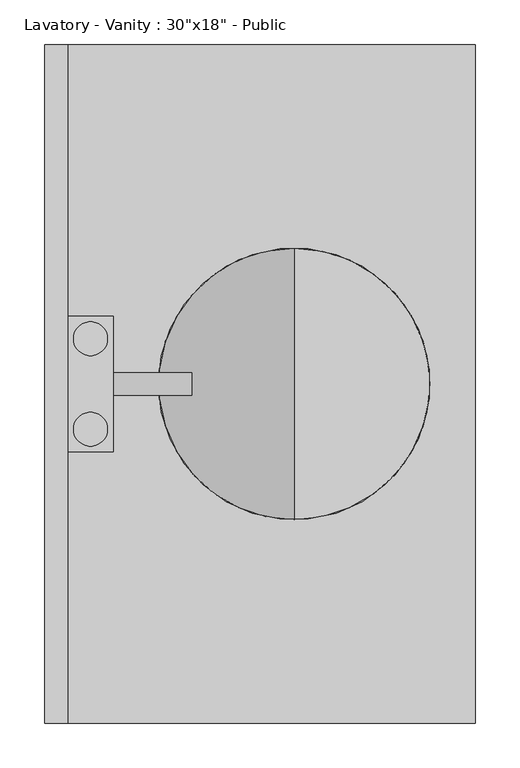
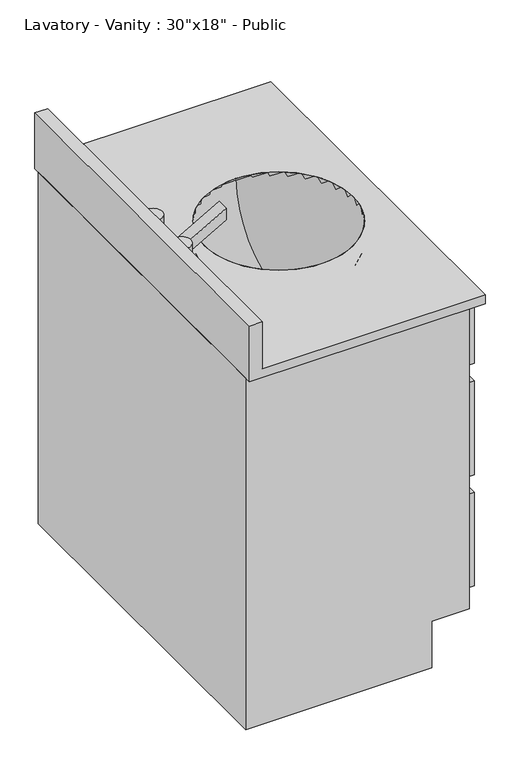
"""IFC4 building model written with IfcOpenShell, lengths in millimetres: flow terminal geometry."""

from ifc_helpers import new_model, si_unit, point, frame, origin, place, context, project, spatial, polyline, circle_curve, ellipse_curve, trimmed, faceted_brep, source, transform, mapped, element, save
from ifc_brep_helpers import plane_surface, cylinder_surface, revolved_surface, advanced_brep


def flow_terminal_15267b2a(model_context):
    return source(origin(), model_context, "Body", "SolidModel", [
        advanced_brep(
        [(32.54375, 50.8, 844.55), (70.64375, 50.8, 844.55), (32.54375, -50.8, 844.55), (70.64375, -50.8, 844.55), (32.54375, 50.8, 806.45), (70.64375, 50.8, 806.45), (32.54375, -50.8, 806.45), (70.64375, -50.8, 806.45), (76.99375, 76.2, 806.45), (26.19375, 76.2, 806.45), (26.19375, -76.2, 806.45), (76.99375, -76.2, 806.45), (76.99375, -12.7, 806.45), (76.99375, 12.7, 806.45), (76.99375, -76.2, 781.05), (26.19375, -76.2, 781.05), (26.19375, 76.2, 781.05), (76.99375, 76.2, 781.05), (76.99375, 12.7, 781.05), (76.99375, -12.7, 781.05), (165.1, -12.7, 831.85), (165.1, -12.7, 857.25), (165.1, 12.7, 857.25), (165.1, 12.7, 831.85)],
        [
            (0, 1, circle_curve(frame((51.59375, 50.8, 844.55), z_axis=(0.0, 0.0, 1.0), x_axis=(1.0, 0.0, 0.0)), 19.05)),
            (1, 0, circle_curve(frame((51.59375, 50.8, 844.55), z_axis=(0.0, 0.0, 1.0), x_axis=(1.0, 0.0, 0.0)), 19.05)),
            (2, 3, circle_curve(frame((51.59375, -50.8, 844.55), z_axis=(0.0, 0.0, 1.0), x_axis=(1.0, 0.0, 0.0)), 19.05)),
            (3, 2, circle_curve(frame((51.59375, -50.8, 844.55), z_axis=(0.0, 0.0, 1.0), x_axis=(1.0, 0.0, 0.0)), 19.05)),
            (0, 4),
            (4, 5, circle_curve(frame((51.59375, 50.8, 806.45), z_axis=(0.0, 0.0, 1.0), x_axis=(1.0, 0.0, 0.0)), 19.05)),
            (5, 1),
            (5, 4, circle_curve(frame((51.59375, 50.8, 806.45), z_axis=(0.0, 0.0, 1.0), x_axis=(1.0, 0.0, 0.0)), 19.05)),
            (2, 6),
            (6, 7, circle_curve(frame((51.59375, -50.8, 806.45), z_axis=(0.0, 0.0, 1.0), x_axis=(1.0, 0.0, 0.0)), 19.05)),
            (7, 3),
            (7, 6, circle_curve(frame((51.59375, -50.8, 806.45), z_axis=(0.0, 0.0, 1.0), x_axis=(1.0, 0.0, 0.0)), 19.05)),
            (8, 9),
            (9, 10),
            (10, 11),
            (11, 12),
            (12, 13),
            (13, 8),
            (14, 15),
            (15, 16),
            (16, 17),
            (17, 18),
            (18, 19),
            (19, 14),
            (8, 17),
            (16, 9),
            (15, 10),
            (14, 11),
            (13, 18),
            (19, 12),
            (19, 20),
            (20, 21),
            (21, 12),
            (13, 22),
            (22, 23),
            (23, 18),
            (23, 20),
            (22, 21),
        ],
        [
            plane_surface(frame((70.64375, 50.8, 844.55), z_axis=(0.0, 0.0, 1.0), x_axis=(0.0, 1.0, 0.0))),
            cylinder_surface(frame((51.59375, 50.8, 806.45), z_axis=(0.0, 0.0, 1.0), x_axis=(1.0, 0.0, 0.0)), 19.05),
            cylinder_surface(frame((51.59375, -50.8, 0.0), z_axis=(0.0, 0.0, 1.0), x_axis=(1.0, 0.0, 0.0)), 19.05),
            plane_surface(frame((26.19375, 76.2, 806.45), z_axis=(0.0, 0.0, 1.0), x_axis=(-1.0, 0.0, 0.0))),
            plane_surface(frame((26.19375, 76.2, 781.05), z_axis=(0.0, 0.0, -1.0), x_axis=(1.0, 0.0, 0.0))),
            plane_surface(frame((76.99375, 76.2, 806.45), z_axis=(0.0, 1.0, 0.0), x_axis=(0.0, 0.0, -1.0))),
            plane_surface(frame((26.19375, 76.2, 806.45), z_axis=(-1.0, 0.0, 0.0), x_axis=(0.0, 0.0, -1.0))),
            plane_surface(frame((26.19375, -76.2, 806.45), z_axis=(0.0, -1.0, 0.0), x_axis=(0.0, 0.0, -1.0))),
            plane_surface(frame((76.99375, -76.2, 806.45), z_axis=(1.0, 0.0, 0.0), x_axis=(0.0, 0.0, -1.0))),
            plane_surface(frame((76.99375, -12.7, 806.45), z_axis=(0.0, -1.0, 0.0), x_axis=(0.0, 0.0, -1.0))),
            plane_surface(frame((76.99375, 12.7, 806.45), z_axis=(0.0, 1.0, 0.0), x_axis=(0.0, 0.0, 1.0))),
            plane_surface(frame((76.99375, -12.7, 781.05), z_axis=(0.4994972193446417, 0.0, -0.8663154897997444), x_axis=(0.0, 1.0, 0.0))),
            plane_surface(frame((165.1, -12.7, 831.85), z_axis=(1.0, 0.0, 0.0), x_axis=(0.0, 1.0, 0.0))),
            plane_surface(frame((165.1, -12.7, 857.25), z_axis=(-0.4994972193446448, 0.0, 0.8663154897997426), x_axis=(0.0, 1.0, 0.0))),
        ],
        [
            (0, [[1, 2]]),
            (0, [[3, 4]]),
            (1, [[-1, 5, 6, 7]]),
            (1, [[-2, -7, 8, -5]]),
            (2, [[-3, 9, 10, 11]]),
            (2, [[-4, -11, 12, -9]]),
            (3, [[13, 14, 15, 16, 17, 18], [-6, -8], [-10, -12]]),
            (4, [[19, 20, 21, 22, 23, 24]]),
            (5, [[-13, 25, -21, 26]]),
            (6, [[-14, -26, -20, 27]]),
            (7, [[-15, -27, -19, 28]]),
            (8, [[-25, -18, 29, -22]]),
            (8, [[-28, -24, 30, -16]]),
            (9, [[31, 32, 33, -30]]),
            (10, [[34, 35, 36, -29]]),
            (11, [[-31, -23, -36, 37]]),
            (12, [[-32, -37, -35, 38]]),
            (13, [[-33, -38, -34, -17]]),
        ],
    ),
        faceted_brep([(381.79375, 368.3, 0.0), (381.79375, -368.3, 0.0), (0.0, -368.3, 0.0), (0.0, 368.3, 0.0), (0.0, 368.3, 762.0), (457.99375, 368.3, 762.0), (457.99375, 368.3, 101.6), (381.79375, 368.3, 101.6), (0.0, -368.3, 762.0), (381.79375, -368.3, 101.6), (457.99375, -368.3, 101.6), (457.99375, -368.3, 762.0), (26.19375, 342.9, 762.0), (445.29375, 342.9, 762.0), (445.29375, -342.9, 762.0), (26.19375, -342.9, 762.0), (457.99375, -342.9, 736.6), (457.99375, 342.9, 736.6), (457.99375, 342.9, 609.6), (457.99375, -342.9, 609.6), (457.99375, -342.9, 571.5), (457.99375, -88.9, 571.5), (457.99375, -88.9, 368.3), (457.99375, -342.9, 368.3), (457.99375, -342.9, 330.2), (457.99375, -88.9, 330.2), (457.99375, -88.9, 127.0), (457.99375, -342.9, 127.0), (457.99375, -50.8, 571.5), (457.99375, 342.9, 571.5), (457.99375, 342.9, 127.0), (457.99375, -50.8, 127.0), (445.29375, 342.9, 368.3), (26.19375, 342.9, 368.3), (26.19375, -342.9, 368.3), (445.29375, -342.9, 368.3), (483.39375, 342.9, 736.6), (483.39375, -342.9, 736.6), (483.39375, -342.9, 609.6), (483.39375, 342.9, 609.6), (483.39375, -88.9, 571.5), (483.39375, -342.9, 571.5), (483.39375, -342.9, 368.3), (483.39375, -88.9, 368.3), (483.39375, -88.9, 330.2), (483.39375, -342.9, 330.2), (483.39375, -342.9, 127.0), (483.39375, -88.9, 127.0), (483.39375, 342.9, 571.5), (483.39375, -50.8, 571.5), (483.39375, -50.8, 127.0), (483.39375, 342.9, 127.0)], [[[0, 1, 2, 3]], [[0, 3, 4, 5, 6, 7]], [[3, 2, 8, 4]], [[2, 1, 9, 10, 11, 8]], [[1, 0, 7, 9]], [[5, 4, 8, 11], [12, 13, 14, 15]], [[6, 10, 9, 7]], [[5, 11, 10, 6], [16, 17, 18, 19], [20, 21, 22, 23], [24, 25, 26, 27], [28, 29, 30, 31]], [[32, 33, 34, 35]], [[33, 32, 13, 12]], [[34, 33, 12, 15]], [[35, 34, 15, 14]], [[32, 35, 14, 13]], [[36, 37, 38, 39]], [[40, 41, 42, 43]], [[44, 45, 46, 47]], [[48, 49, 50, 51]], [[37, 36, 17, 16]], [[38, 37, 16, 19]], [[39, 38, 19, 18]], [[36, 39, 18, 17]], [[41, 40, 21, 20]], [[42, 41, 20, 23]], [[43, 42, 23, 22]], [[40, 43, 22, 21]], [[45, 44, 25, 24]], [[46, 45, 24, 27]], [[47, 46, 27, 26]], [[44, 47, 26, 25]], [[49, 48, 29, 28]], [[50, 49, 28, 31]], [[51, 50, 31, 30]], [[48, 51, 30, 29]]]),
        advanced_brep(
        [(483.39375, -381.0, 781.05), (483.39375, 381.0, 781.05), (26.19375, 381.0, 781.05), (26.19375, -381.0, 781.05), (432.59375, 0.0, 781.05), (127.79375, 0.0, 781.05), (483.39375, 381.0, 762.0), (483.39375, -381.0, 762.0), (0.0, -381.0, 762.0), (0.0, 381.0, 762.0), (127.79375, 0.0, 762.0), (432.59375, 0.0, 762.0), (0.0, 381.0, 882.65), (26.19375, 381.0, 882.65), (0.0, -381.0, 882.65), (26.19375, -381.0, 882.65)],
        [
            (0, 1),
            (1, 2),
            (2, 3),
            (3, 0),
            (4, 5, circle_curve(frame((280.19375, 0.0, 781.05), z_axis=(0.0, 0.0, -1.0), x_axis=(1.0, 0.0, 0.0)), 152.4)),
            (5, 4, circle_curve(frame((280.19375, 0.0, 781.05), z_axis=(0.0, 0.0, -1.0), x_axis=(1.0, 0.0, 0.0)), 152.4)),
            (6, 7),
            (7, 8),
            (8, 9),
            (9, 6),
            (10, 11, circle_curve(frame((280.19375, 0.0, 762.0), z_axis=(0.0, 0.0, 1.0), x_axis=(1.0, 0.0, 0.0)), 152.4)),
            (11, 10, circle_curve(frame((280.19375, 0.0, 762.0), z_axis=(0.0, 0.0, 1.0), x_axis=(1.0, 0.0, 0.0)), 152.4)),
            (9, 12),
            (12, 13),
            (13, 2),
            (1, 6),
            (8, 14),
            (14, 12),
            (7, 0),
            (3, 15),
            (15, 14),
            (4, 11),
            (10, 5),
            (15, 13),
        ],
        [
            plane_surface(frame((0.0, 381.0, 781.05), z_axis=(0.0, 0.0, 1.0), x_axis=(-1.0, 0.0, 0.0))),
            plane_surface(frame((0.0, 381.0, 762.0), z_axis=(0.0, 0.0, -1.0), x_axis=(1.0, 0.0, 0.0))),
            plane_surface(frame((483.39375, 381.0, 781.05), z_axis=(0.0, 1.0, 0.0), x_axis=(0.0, 0.0, -1.0))),
            plane_surface(frame((0.0, 381.0, 781.05), z_axis=(-1.0, 0.0, 0.0), x_axis=(0.0, 0.0, -1.0))),
            plane_surface(frame((0.0, -381.0, 781.05), z_axis=(0.0, -1.0, 0.0), x_axis=(0.0, 0.0, -1.0))),
            plane_surface(frame((483.39375, -381.0, 781.05), z_axis=(1.0, 0.0, 0.0), x_axis=(0.0, 0.0, -1.0))),
            revolved_surface(polyline([(432.59375, 0.0, 781.05), (432.59375, 0.0, 762.0)]), (280.19375, 0.0, 762.0), (0.0, 0.0, 1.0)),
            plane_surface(frame((0.0, 381.0, 882.65), z_axis=(0.0, 0.0, 1.0), x_axis=(-1.0, 0.0, 0.0))),
            plane_surface(frame((26.19375, -381.0, 882.65), z_axis=(1.0, 0.0, 0.0), x_axis=(0.0, 0.0, -1.0))),
        ],
        [
            (0, [[1, 2, 3, 4], [5, 6]]),
            (1, [[7, 8, 9, 10], [11, 12]]),
            (2, [[-10, 13, 14, 15, -2, 16]]),
            (3, [[-13, -9, 17, 18]]),
            (4, [[-17, -8, 19, -4, 20, 21]]),
            (5, [[-1, -19, -7, -16]]),
            (6, [[22, -11, 23, -5]]),
            (6, [[-22, -6, -23, -12]]),
            (7, [[-14, -18, -21, 24]]),
            (8, [[-24, -20, -3, -15]]),
        ],
    ),
        advanced_brep(
        [(280.19375, 0.0, 628.65), (280.19375, 152.4, 781.05), (280.19375, -152.4, 781.05), (280.19375, -44.45, 628.65), (280.19375, 44.45, 628.65), (280.19375, 0.0, 628.65), (280.19375, -157.6028553, 762.0), (280.19375, 157.6028553, 762.0)],
        [
            (0, 1, circle_curve(frame((280.19375, 0.0, 781.05), z_axis=(1.0, 0.0, 0.0), x_axis=(0.0, 1.0, 0.0)), 152.4)),
            (1, 2, circle_curve(frame((280.19375, 0.0, 781.05), z_axis=(0.0, 0.0, 1.0), x_axis=(0.0, 1.0, 0.0)), 152.4)),
            (2, 0, circle_curve(frame((280.19375, 0.0, 781.05), z_axis=(1.0, 0.0, 0.0), x_axis=(0.0, -1.0, 0.0)), 152.4)),
            (2, 1, circle_curve(frame((280.19375, 0.0, 781.05), z_axis=(0.0, 0.0, 1.0), x_axis=(0.0, 1.0, 0.0)), 152.4)),
            (3, 4, circle_curve(frame((280.19375, 0.0, 628.65), z_axis=(0.0, 0.0, -1.0), x_axis=(0.0, 1.0, 0.0)), 44.45)),
            (4, 5),
            (5, 3),
            (4, 3, circle_curve(frame((280.19375, 0.0, 628.65), z_axis=(0.0, 0.0, -1.0), x_axis=(0.0, 1.0, 0.0)), 44.45)),
            (6, 7, circle_curve(frame((280.19375, 0.0, 762.0), z_axis=(0.0, 0.0, -1.0), x_axis=(0.0, 1.0, 0.0)), 157.6028553)),
            (7, 4, circle_curve(frame((280.19375, 0.0, 781.05), z_axis=(-1.0, 0.0, 0.0), x_axis=(0.0, 1.0, 0.0)), 158.75)),
            (3, 6, circle_curve(frame((280.19375, 0.0, 781.05), z_axis=(-1.0, 0.0, 0.0), x_axis=(0.0, -1.0, 0.0)), 158.75)),
            (7, 6, circle_curve(frame((280.19375, 0.0, 762.0), z_axis=(0.0, 0.0, -1.0), x_axis=(0.0, 1.0, 0.0)), 157.6028553)),
            (1, 7),
            (6, 2),
        ],
        [
            revolved_surface(trimmed(ellipse_curve(frame((280.19375, 0.0, 781.05), z_axis=(-1.0, 0.0, 0.0), x_axis=(0.0, 1.0, 0.0)), 152.4, 152.4), [point((280.19375, 152.4, 781.05))], [point((280.19375, 0.0, 628.65))], True, "CARTESIAN"), (280.19375, 0.0, 520.7), (0.0, 0.0, 1.0)),
            plane_surface(frame((280.19375, 0.0, 628.65), z_axis=(0.0, 0.0, -1.0), x_axis=(0.0, 1.0, 0.0))),
            revolved_surface(trimmed(ellipse_curve(frame((280.19375, 0.0, 781.05), z_axis=(1.0, 0.0, 0.0), x_axis=(0.0, 1.0, 0.0)), 158.75, 158.75), [point((280.19375, 44.45, 628.65))], [point((280.19375, 157.6028553, 762.0))], True, "CARTESIAN"), (280.19375, 0.0, 520.7), (0.0, 0.0, 1.0)),
            revolved_surface(polyline([(280.19375, 157.6028553, 762.0), (280.19375, 152.4, 781.05)]), (280.19375, 0.0, 520.7), (0.0, 0.0, 1.0)),
        ],
        [
            (0, [[1, 2, 3]]),
            (0, [[-3, 4, -1]]),
            (1, [[5, 6, 7]]),
            (1, [[8, -7, -6]]),
            (2, [[9, 10, -5, 11]]),
            (2, [[12, -11, -8, -10]]),
            (3, [[-2, 13, -9, 14]]),
            (3, [[-4, -14, -12, -13]]),
        ],
    ),
    ])


if __name__ == "__main__":
    model = new_model("IFC4")
    model_context = context("Model", 3, world=origin())
    ifc_project = project(units=[si_unit("LENGTHUNIT", "METRE", prefix="MILLI")], contexts=[model_context])
    site = spatial("IfcSite", under=ifc_project)
    building = spatial("IfcBuilding", under=site)
    placement = place(None, origin())
    flow_terminal_shape = flow_terminal_15267b2a(model_context)
    element("IfcFlowTerminal", 1, ObjectType="Lavatory - Vanity : 30\"x18\" - Public", at=placement, inside=building, context=model_context, shape_type="MappedRepresentation", body=[
        mapped(flow_terminal_shape, transform((0.0, 0.0, 0.0), x_axis=(1.0, 0.0, 0.0), y_axis=(0.0, 1.0, 0.0), z_axis=(0.0, 0.0, 1.0))),
    ])
    save(model, "model.ifc")

# Revit data of these elements
# Type "Lavatory - Vanity : 30\"x18\" - Public"
#   Sanitary Radius = 5/8"
#   Sanitary Diameter = 1 1/4"
#   WFU = 1
#   Lavatory Length = 1' - 6"
#   Lavatory Width = 2' - 6"
#   Hot Water Radius = 1/4"
#   Hot Water Diameter = 1/2"
#   Half Lavatory Width = 1' - 3"
#   HWFU = 1.5
#   Flow Pressure [instance default] = 8.00 psi
#   Cold Water Radius = 1/4"
#   Cold Water Diameter = 1/2"
#   CWFU = 1.5
#   Sink Material = none
#   Faucet Material = none
#   Cabinet Top Material = none
#   Cabinet Material = none
#   Default Elevation = 0
